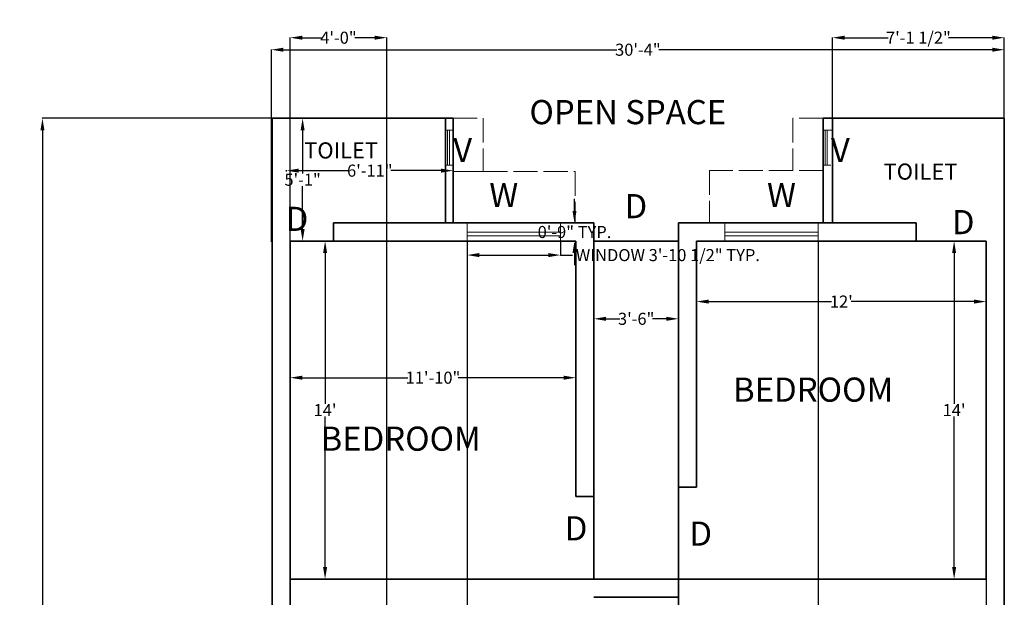
# Model space of a CAD drawing. Units: inches. Extents: x -732 to -187, y 754 to 1605.
# Tile 2 of 2: x -732 to -242, y 1318 to 1605. Entities that reach past the tile are written whole.
import ezdxf

# ---------------------------------------------------------------- set-up
doc = ezdxf.new("R2010")
doc.units = ezdxf.units.IN
doc.header["$MEASUREMENT"] = 0
doc.linetypes.add('ACAD_ISO02W100', pattern=[15, 12, -3])
for name, color, linetype, lineweight in [('A-ANNO-DIMS', 2, 'Continuous', 18), ('A-ANNO-TEXT', 3, 'Continuous', 18), ('A-AREA-IDEN', 7, 'Continuous', 25), ('A-GLAZ', 4, 'Continuous', 18), ('A-ROOF', 8, 'Continuous', 18), ('A-ROOF-OVHD', 8, 'ACAD_ISO02W100', 18), ('A-WALL', 7, 'Continuous', 35)]:
    doc.layers.add(name, color=color, linetype=linetype, lineweight=lineweight)
doc.styles.get("Standard").update_dxf_attribs({"font": 'arial.ttf'})
doc.dimstyles.get("Standard").update_dxf_attribs({"dimtxt": 6, "dimasz": 6, "dimexe": 0.18, "dimexo": 0.0625, "dimgap": 0.09, "dimtad": 0, "dimtih": 1, "dimtoh": 1, "dimdec": 0, "dimzin": 0, "dimdsep": 46, "dimlunit": 3, "dimtxsty": 'Standard', "dimcen": 0.09, "dimadec": 0, "dimazin": 0, "dimtfac": 1, "dimtdec": 0, "dimtofl": 0, "dimtmove": 0, "dimatfit": 3, "dimfxl": 1, "dimtolj": 1, "dimtzin": 0, "dimarcsym": 0})

# ---------------------------------------------------------------- blocks, each defined once
blk = doc.blocks.new('*D1')
at = {"layer": 'A-ANNO-DIMS', "color": 0, "lineweight": -2, "transparency": 16777216}
for p, q in [((-446.28, 1440.67), (-446.28, 1456.43)), ((-440.28, 1456.25), (-433.34, 1456.25)), ((-410.28, 1456.25), (-417.22, 1456.25)), ((-404.28, 1440.67), (-404.28, 1456.43))]:
    blk.add_line(p, q, dxfattribs=at)
at = {"layer": 'A-ANNO-DIMS', "color": 0, "transparency": 16777216}
for points in [[(-440.28, 1457.25), (-440.28, 1455.25), (-446.28, 1456.25)], [(-410.28, 1457.25), (-410.28, 1455.25), (-404.28, 1456.25)]]:
    blk.add_solid(points, dxfattribs=at)
at = {"layer": 'Defpoints', "color": 0, "transparency": 16777216}
for p in [(-404.28, 1456.25), (-446.28, 1440.61), (-404.28, 1440.61)]:
    blk.add_point(p, dxfattribs=at)
at = {"layer": 'A-ANNO-DIMS', "color": 0, "transparency": 16777216, "insert": (-425.28, 1456.25), "char_height": 6, "attachment_point": 5}
blk.add_mtext('\\A1;3\'-6"', dxfattribs=at)
blk = doc.blocks.new('*D2')
at = {"layer": 'A-ANNO-DIMS', "color": 0, "lineweight": -2, "transparency": 16777216}
for p, q in [((-395.28, 1479.29), (-395.28, 1464.63)), ((-251.28, 1479.29), (-251.28, 1464.63)), ((-389.28, 1464.81), (-328.18, 1464.81)), ((-257.28, 1464.81), (-318.38, 1464.81))]:
    blk.add_line(p, q, dxfattribs=at)
at = {"layer": 'A-ANNO-DIMS', "color": 0, "transparency": 16777216}
for points in [[(-389.28, 1465.81), (-389.28, 1463.81), (-395.28, 1464.81)], [(-257.28, 1465.81), (-257.28, 1463.81), (-251.28, 1464.81)]]:
    blk.add_solid(points, dxfattribs=at)
at = {"layer": 'Defpoints', "color": 0, "transparency": 16777216}
for p in [(-395.28, 1479.35), (-251.28, 1479.35), (-251.28, 1464.81)]:
    blk.add_point(p, dxfattribs=at)
at = {"layer": 'A-ANNO-DIMS', "color": 0, "transparency": 16777216, "insert": (-323.28, 1464.81), "char_height": 6, "attachment_point": 5}
blk.add_mtext("\\A1;12'", dxfattribs=at)
blk = doc.blocks.new('*D3')
at = {"layer": 'A-ANNO-DIMS', "color": 0, "lineweight": -2, "transparency": 16777216}
for p, q in [((-597.28, 1427.05), (-597.28, 1427.17)), ((-591.28, 1426.99), (-538.72, 1426.99)), ((-461.28, 1426.99), (-513.83, 1426.99)), ((-455.28, 1427.05), (-455.28, 1427.17))]:
    blk.add_line(p, q, dxfattribs=at)
at = {"layer": 'A-ANNO-DIMS', "color": 0, "transparency": 16777216}
for points in [[(-591.28, 1427.99), (-591.28, 1425.99), (-597.28, 1426.99)], [(-461.28, 1427.99), (-461.28, 1425.99), (-455.28, 1426.99)]]:
    blk.add_solid(points, dxfattribs=at)
at = {"layer": 'Defpoints', "color": 0, "transparency": 16777216}
for p in [(-597.28, 1426.99), (-455.28, 1426.99), (-455.28, 1426.99)]:
    blk.add_point(p, dxfattribs=at)
at = {"layer": 'A-ANNO-DIMS', "color": 0, "transparency": 16777216, "insert": (-526.28, 1426.99), "char_height": 6, "attachment_point": 5}
blk.add_mtext('\\A1;11\'-10"', dxfattribs=at)
blk = doc.blocks.new('*D19')
at = {"layer": 'A-ANNO-DIMS', "color": 0, "lineweight": -2, "transparency": 16777216}
for p, q in [((-251.34, 1494.88), (-267.41, 1494.88)), ((-267.23, 1488.88), (-267.23, 1413.98)), ((-267.23, 1332.88), (-267.23, 1407.78)), ((-251.34, 1326.88), (-267.41, 1326.88))]:
    blk.add_line(p, q, dxfattribs=at)
at = {"layer": 'A-ANNO-DIMS', "color": 0, "transparency": 16777216}
for points in [[(-268.23, 1488.88), (-266.23, 1488.88), (-267.23, 1494.88)], [(-268.23, 1332.88), (-266.23, 1332.88), (-267.23, 1326.88)]]:
    blk.add_solid(points, dxfattribs=at)
at = {"layer": 'Defpoints', "color": 0, "transparency": 16777216}
for p in [(-251.28, 1494.88), (-267.23, 1326.88), (-251.28, 1326.88)]:
    blk.add_point(p, dxfattribs=at)
at = {"layer": 'A-ANNO-DIMS', "color": 0, "transparency": 16777216, "insert": (-267.23, 1410.88), "char_height": 6, "attachment_point": 5}
blk.add_mtext("\\A1;14'", dxfattribs=at)
blk = doc.blocks.new('*D20')
at = {"layer": 'A-ANNO-DIMS', "color": 0, "lineweight": -2, "transparency": 16777216}
for p, q in [((-597.22, 1494.88), (-579.74, 1494.88)), ((-579.92, 1488.88), (-579.92, 1413.98)), ((-579.92, 1332.88), (-579.92, 1407.77)), ((-597.22, 1326.88), (-579.74, 1326.88))]:
    blk.add_line(p, q, dxfattribs=at)
at = {"layer": 'A-ANNO-DIMS', "color": 0, "transparency": 16777216}
for points in [[(-580.92, 1488.88), (-578.92, 1488.88), (-579.92, 1494.88)], [(-580.92, 1332.88), (-578.92, 1332.88), (-579.92, 1326.88)]]:
    blk.add_solid(points, dxfattribs=at)
at = {"layer": 'Defpoints', "color": 0, "transparency": 16777216}
for p in [(-597.28, 1494.88), (-597.28, 1326.88), (-579.92, 1326.88)]:
    blk.add_point(p, dxfattribs=at)
at = {"layer": 'A-ANNO-DIMS', "color": 0, "transparency": 16777216, "insert": (-579.92, 1410.88), "char_height": 6, "attachment_point": 5}
blk.add_mtext("\\A1;14'", dxfattribs=at)
blk = doc.blocks.new('*D21')
at = {"layer": 'A-ANNO-DIMS', "color": 0, "lineweight": -2, "transparency": 16777216}
for p, q in [((-584.99, 1555.88), (-591.28, 1555.88)), ((-591.1, 1549.88), (-591.1, 1528.53)), ((-591.1, 1500.88), (-591.1, 1522.22)), ((-584.99, 1494.88), (-591.28, 1494.88))]:
    blk.add_line(p, q, dxfattribs=at)
at = {"layer": 'A-ANNO-DIMS', "color": 0, "transparency": 16777216}
for points in [[(-592.1, 1549.88), (-590.1, 1549.88), (-591.1, 1555.88)], [(-592.1, 1500.88), (-590.1, 1500.88), (-591.1, 1494.88)]]:
    blk.add_solid(points, dxfattribs=at)
at = {"layer": 'Defpoints', "color": 0, "transparency": 16777216}
for p in [(-584.93, 1555.88), (-591.1, 1494.88), (-584.93, 1494.88)]:
    blk.add_point(p, dxfattribs=at)
at = {"layer": 'A-ANNO-DIMS', "color": 0, "transparency": 16777216, "insert": (-591.1, 1525.38), "char_height": 6, "attachment_point": 5}
blk.add_mtext('\\A1;5\'-1"', dxfattribs=at)
blk = doc.blocks.new('*D22')
at = {"layer": 'A-ANNO-DIMS', "color": 0, "lineweight": -2, "transparency": 16777216}
for p, q in [((-599.1, 1529.44), (-599.1, 1530.06)), ((-593.1, 1529.88), (-568.1, 1529.88)), ((-522.28, 1529.88), (-547.28, 1529.88)), ((-516.28, 1529.44), (-516.28, 1530.06))]:
    blk.add_line(p, q, dxfattribs=at)
at = {"layer": 'A-ANNO-DIMS', "color": 0, "transparency": 16777216}
for points in [[(-593.1, 1530.88), (-593.1, 1528.88), (-599.1, 1529.88)], [(-522.28, 1530.88), (-522.28, 1528.88), (-516.28, 1529.88)]]:
    blk.add_solid(points, dxfattribs=at)
at = {"layer": 'Defpoints', "color": 0, "transparency": 16777216}
for p in [(-599.1, 1529.88), (-599.1, 1529.38), (-516.28, 1529.38)]:
    blk.add_point(p, dxfattribs=at)
at = {"layer": 'A-ANNO-DIMS', "color": 0, "transparency": 16777216, "insert": (-557.69, 1529.88), "char_height": 6, "attachment_point": 5}
blk.add_mtext('\\A1;6\'-11"', dxfattribs=at)
blk = doc.blocks.new('*D23')
at = {"layer": 'A-ANNO-DIMS', "color": 0, "lineweight": -2, "transparency": 16777216}
for p, q in [((-606.6, 1494.55), (-606.6, 1590.14)), ((-600.6, 1589.96), (-434.83, 1589.96)), ((-248.28, 1589.96), (-414.04, 1589.96)), ((-242.28, 1494.55), (-242.28, 1590.14))]:
    blk.add_line(p, q, dxfattribs=at)
at = {"layer": 'A-ANNO-DIMS', "color": 0, "transparency": 16777216}
for points in [[(-600.6, 1590.96), (-600.6, 1588.96), (-606.6, 1589.96)], [(-248.28, 1590.96), (-248.28, 1588.96), (-242.28, 1589.96)]]:
    blk.add_solid(points, dxfattribs=at)
at = {"layer": 'Defpoints', "color": 0, "transparency": 16777216}
for p in [(-242.28, 1589.96), (-606.6, 1494.48), (-242.28, 1494.48)]:
    blk.add_point(p, dxfattribs=at)
at = {"layer": 'A-ANNO-DIMS', "color": 0, "transparency": 16777216, "insert": (-424.44, 1589.96), "char_height": 6, "attachment_point": 5}
blk.add_mtext('\\A1;30\'-4"', dxfattribs=at)
blk = doc.blocks.new('*D24')
at = {"layer": 'A-ANNO-DIMS', "color": 0, "lineweight": -2, "transparency": 16777216}
for p, q in [((-606.34, 1555.88), (-720.61, 1555.88)), ((-720.43, 1549.88), (-720.43, 1197.03)), ((-720.43, 837.88), (-720.43, 1190.72)), ((-606.34, 831.88), (-720.61, 831.88))]:
    blk.add_line(p, q, dxfattribs=at)
at = {"layer": 'A-ANNO-DIMS', "color": 0, "transparency": 16777216}
for points in [[(-721.43, 1549.88), (-719.43, 1549.88), (-720.43, 1555.88)], [(-721.43, 837.88), (-719.43, 837.88), (-720.43, 831.88)]]:
    blk.add_solid(points, dxfattribs=at)
at = {"layer": 'Defpoints', "color": 0, "transparency": 16777216}
for p in [(-606.28, 1555.88), (-720.43, 831.88), (-606.28, 831.88)]:
    blk.add_point(p, dxfattribs=at)
at = {"layer": 'A-ANNO-DIMS', "color": 0, "transparency": 16777216, "insert": (-720.43, 1193.88), "char_height": 6, "attachment_point": 5}
blk.add_mtext('\\A1;60\'-4"', dxfattribs=at)
blk = doc.blocks.new('WIN-REAR-BEDROOM')
for p, q in [((0, 9), (0, 0)), ((46.43, 9), (46.43, 0)), ((0, 4.5), (46.43, 4.5)), ((0, 2.55), (46.43, 2.55))]:
    blk.add_line(p, q)
blk = doc.blocks.new('*D26')
at = {"layer": 'A-ANNO-DIMS', "color": 0, "lineweight": -2, "transparency": 16777216}
for p, q in [((-509.33, 1494.81), (-509.33, 1487.73)), ((-462.9, 1494.81), (-462.9, 1487.73)), ((-503.33, 1487.91), (-468.9, 1487.91)), ((-462.9, 1487.91), (-456.9, 1487.91))]:
    blk.add_line(p, q, dxfattribs=at)
at = {"layer": 'A-ANNO-DIMS', "color": 0, "transparency": 16777216}
for points in [[(-503.33, 1488.91), (-503.33, 1486.91), (-509.33, 1487.91)], [(-468.9, 1488.91), (-468.9, 1486.91), (-462.9, 1487.91)]]:
    blk.add_solid(points, dxfattribs=at)
at = {"layer": 'Defpoints', "color": 0, "transparency": 16777216}
for p in [(-509.33, 1494.88), (-462.9, 1494.88), (-462.9, 1487.91)]:
    blk.add_point(p, dxfattribs=at)
at = {"layer": 'A-ANNO-DIMS', "color": 0, "transparency": 16777216, "insert": (-409.53, 1487.91), "char_height": 6, "attachment_point": 5}
blk.add_mtext('\\A1;WINDOW 3\'-10 1/2" TYP.', dxfattribs=at)
blk = doc.blocks.new('*D27')
at = {"layer": 'A-ANNO-DIMS', "color": 0, "lineweight": -2, "transparency": 16777216}
for p, q in [((-455.94, 1509.88), (-455.94, 1515.88)), ((-462.84, 1503.88), (-455.76, 1503.88)), ((-462.84, 1494.88), (-455.76, 1494.88)), ((-455.94, 1488.88), (-455.94, 1482.88))]:
    blk.add_line(p, q, dxfattribs=at)
at = {"layer": 'A-ANNO-DIMS', "color": 0, "transparency": 16777216}
for points in [[(-456.94, 1509.88), (-454.94, 1509.88), (-455.94, 1503.88)], [(-456.94, 1488.88), (-454.94, 1488.88), (-455.94, 1494.88)]]:
    blk.add_solid(points, dxfattribs=at)
at = {"layer": 'Defpoints', "color": 0, "transparency": 16777216}
for p in [(-462.9, 1503.88), (-455.94, 1503.88), (-462.9, 1494.88)]:
    blk.add_point(p, dxfattribs=at)
at = {"layer": 'A-ANNO-DIMS', "color": 0, "transparency": 16777216, "insert": (-455.94, 1499.38), "char_height": 6, "attachment_point": 5}
blk.add_mtext('\\A1;0\'-9" TYP.', dxfattribs=at)
blk = doc.blocks.new('*D33')
at = {"layer": 'A-ANNO-DIMS', "color": 0, "lineweight": -2, "transparency": 16777216}
for p, q in [((-597.28, 1084.94), (-597.28, 1596.11)), ((-591.28, 1595.93), (-581.46, 1595.93)), ((-555.28, 1595.93), (-565.09, 1595.93)), ((-549.28, 1084.94), (-549.28, 1596.11))]:
    blk.add_line(p, q, dxfattribs=at)
at = {"layer": 'A-ANNO-DIMS', "color": 0, "transparency": 16777216}
for points in [[(-591.28, 1596.93), (-591.28, 1594.93), (-597.28, 1595.93)], [(-555.28, 1596.93), (-555.28, 1594.93), (-549.28, 1595.93)]]:
    blk.add_solid(points, dxfattribs=at)
at = {"layer": 'Defpoints', "color": 0, "transparency": 16777216}
for p in [(-549.28, 1595.93), (-597.28, 1084.88), (-549.28, 1084.88)]:
    blk.add_point(p, dxfattribs=at)
at = {"layer": 'A-ANNO-DIMS', "color": 0, "transparency": 16777216, "insert": (-573.28, 1595.93), "char_height": 6, "attachment_point": 5}
blk.add_mtext('\\A1;4\'-0"', dxfattribs=at)
blk = doc.blocks.new('*D36')
at = {"layer": 'A-ANNO-DIMS', "color": 0, "lineweight": -2, "transparency": 16777216}
for p, q in [((-327.69, 1555.94), (-327.69, 1596.11)), ((-321.69, 1595.93), (-300.02, 1595.93)), ((-248.28, 1595.93), (-269.95, 1595.93)), ((-242.28, 1555.94), (-242.28, 1596.11))]:
    blk.add_line(p, q, dxfattribs=at)
at = {"layer": 'A-ANNO-DIMS', "color": 0, "transparency": 16777216}
for points in [[(-321.69, 1596.93), (-321.69, 1594.93), (-327.69, 1595.93)], [(-248.28, 1596.93), (-248.28, 1594.93), (-242.28, 1595.93)]]:
    blk.add_solid(points, dxfattribs=at)
at = {"layer": 'Defpoints', "color": 0, "transparency": 16777216}
for p in [(-242.28, 1595.93), (-327.69, 1555.88), (-242.28, 1555.88)]:
    blk.add_point(p, dxfattribs=at)
at = {"layer": 'A-ANNO-DIMS', "color": 0, "transparency": 16777216, "insert": (-284.98, 1595.93), "char_height": 6, "attachment_point": 5}
blk.add_mtext('\\A1;7\'-1 1/2"', dxfattribs=at)
blk = doc.blocks.new('*D37')
at = {"layer": 'A-ANNO-DIMS', "color": 0, "lineweight": -2, "transparency": 16777216}
for p, q in [((-597.28, 1494.81), (-597.28, 763.13)), ((-509.33, 1494.81), (-509.33, 763.13)), ((-591.28, 763.31), (-561.35, 763.31)), ((-515.33, 763.31), (-545.27, 763.31))]:
    blk.add_line(p, q, dxfattribs=at)
at = {"layer": 'A-ANNO-DIMS', "color": 0, "transparency": 16777216}
for points in [[(-591.28, 764.31), (-591.28, 762.31), (-597.28, 763.31)], [(-515.33, 764.31), (-515.33, 762.31), (-509.33, 763.31)]]:
    blk.add_solid(points, dxfattribs=at)
at = {"layer": 'Defpoints', "color": 0, "transparency": 16777216}
for p in [(-597.28, 1494.88), (-509.33, 1494.88), (-509.33, 763.31)]:
    blk.add_point(p, dxfattribs=at)
at = {"layer": 'A-ANNO-DIMS', "color": 0, "transparency": 16777216, "insert": (-553.31, 763.31), "char_height": 6, "attachment_point": 5}
blk.add_mtext('\\A1;7\'-4"', dxfattribs=at)
blk = doc.blocks.new('*D38')
at = {"layer": 'A-ANNO-DIMS', "color": 0, "lineweight": -2, "transparency": 16777216}
for p, q in [((-334.82, 1494.81), (-334.82, 763.13)), ((-251.28, 1494.82), (-251.28, 763.13)), ((-328.82, 763.31), (-310.45, 763.31)), ((-257.28, 763.31), (-275.65, 763.31))]:
    blk.add_line(p, q, dxfattribs=at)
at = {"layer": 'A-ANNO-DIMS', "color": 0, "transparency": 16777216}
for points in [[(-328.82, 764.31), (-328.82, 762.31), (-334.82, 763.31)], [(-257.28, 764.31), (-257.28, 762.31), (-251.28, 763.31)]]:
    blk.add_solid(points, dxfattribs=at)
at = {"layer": 'Defpoints', "color": 0, "transparency": 16777216}
for p in [(-334.82, 1494.88), (-251.28, 1494.88), (-251.28, 763.31)]:
    blk.add_point(p, dxfattribs=at)
at = {"layer": 'A-ANNO-DIMS', "color": 0, "transparency": 16777216, "insert": (-293.05, 763.31), "char_height": 6, "attachment_point": 5}
blk.add_mtext('\\A1;6\'-11 1/2"', dxfattribs=at)

msp = doc.modelspace()

# ---------------------------------------------------------------- linework, layer by layer
at = {"layer": 'A-GLAZ'}
for p, q in [((-520, 1549.98), (-516.28, 1549.98)), ((-519.04, 1549.98), (-519.04, 1532.62)), ((-518.05, 1549.98), (-518.14, 1532.62)), ((-332.23, 1549.98), (-327.69, 1549.98)), ((-331.27, 1549.98), (-331.27, 1532.62)), ((-330.28, 1549.98), (-330.37, 1532.62)), ((-520, 1532.62), (-516.28, 1532.62)), ((-332.23, 1532.62), (-328.51, 1532.62))]:
    msp.add_line(p, q, dxfattribs=at)
at = {"layer": 'A-ROOF'}
msp.add_line((-501.27, 1529.38), (-516.28, 1529.38), dxfattribs=at)
at = {"layer": 'A-ROOF-OVHD'}
for p, q in [((-516.28, 1555.88), (-501.27, 1555.88)), ((-501.27, 1555.88), (-501.27, 1529.38)), ((-332.28, 1555.88), (-347.36, 1555.88)), ((-347.36, 1555.88), (-347.36, 1529.88)), ((-516.28, 1529.38), (-455.67, 1529.38)), ((-455.67, 1529.38), (-455.67, 1503.88)), ((-379.11, 1529.88), (-388.9, 1529.88)), ((-388.9, 1529.88), (-388.9, 1503.88)), ((-332.28, 1529.88), (-379.11, 1529.88))]:
    msp.add_line(p, q, dxfattribs=at)
at = {"layer": 'A-WALL'}
for p, q in [((-606.28, 1555.88), (-516.28, 1555.88)), ((-606.28, 1503.88), (-606.28, 1555.88)), ((-516.28, 1555.88), (-520, 1555.88)), ((-520, 1555.88), (-520, 1503.88)), ((-516.28, 1555.88), (-516.28, 1503.88)), ((-242.28, 1555.88), (-332.28, 1555.88)), ((-332.28, 1555.88), (-332.28, 1503.88)), ((-327.69, 1555.88), (-327.69, 1503.88)), ((-242.28, 1503.88), (-242.28, 1555.88)), ((-606.28, 1326.88), (-606.28, 1503.88)), ((-516.28, 1503.88), (-575.75, 1503.88)), ((-575.75, 1503.88), (-575.75, 1494.88)), ((-575.75, 1503.88), (-446.28, 1503.88)), ((-520, 1503.88), (-516.28, 1503.88)), ((-446.28, 1503.88), (-446.28, 1494.88)), ((-404.28, 1503.88), (-286.13, 1503.88)), ((-404.28, 1317.88), (-404.28, 1503.88)), ((-286.13, 1503.88), (-286.13, 1494.88)), ((-242.28, 1503.88), (-242.28, 1326.88)), ((-597.28, 1494.88), (-455.28, 1494.88)), ((-597.28, 1326.88), (-597.28, 1494.88)), ((-455.28, 1494.88), (-588.28, 1494.88)), ((-455.28, 1368.04), (-455.28, 1494.88)), ((-446.28, 1494.88), (-446.28, 1326.88)), ((-446.28, 1494.88), (-404.28, 1494.88)), ((-446.28, 1326.88), (-446.28, 1494.88)), ((-404.28, 1494.88), (-404.28, 1326.88)), ((-395.28, 1372.67), (-395.28, 1494.88)), ((-395.28, 1494.88), (-251.28, 1494.88)), ((-251.28, 1494.88), (-251.28, 1326.88)), ((-404.28, 1372.67), (-395.28, 1372.67)), ((-446.28, 1368.04), (-455.28, 1368.04)), ((-606.28, 1326.88), (-606.28, 831.88)), ((-446.28, 1326.88), (-597.28, 1326.88)), ((-404.28, 1326.88), (-446.28, 1326.88)), ((-251.28, 1326.88), (-404.28, 1326.88)), ((-242.28, 1326.88), (-242.28, 831.88)), ((-404.28, 1317.88), (-446.28, 1317.88)), ((-404.28, 1317.88), (-404.28, 1032.88))]:
    msp.add_line(p, q, dxfattribs=at)

# ---------------------------------------------------------------- block references
at = {"layer": 'A-GLAZ'}
for p in [(-509.33, 1494.88), (-381.25, 1494.88)]:
    msp.add_blockref('WIN-REAR-BEDROOM', p, dxfattribs=at)

# ---------------------------------------------------------------- texts
at = {"layer": 'A-ANNO-TEXT', "char_height": 12}
for s, width, insert, attachment_point in [('V', 35.4038, (-516.26, 1546.14), 1), ('V', 35.4038, (-328.49, 1546.14), 1), ('W', 35.4038, (-498.3, 1523.76), 1), ('W', 35.4038, (-345.85, 1523.76), 3), ('D', 8.414, (-431.06, 1518.24), 1), ('D', 8.414, (-599.52, 1511.9), 1), ('D', 8.414, (-268.34, 1510.3), 1), ('D', 8.414, (-460.77, 1358.15), 1), ('D', 8.414, (-398.83, 1355.51), 1)]:
    msp.add_mtext_dynamic_manual_height_columns(s, width=width, gutter_width=1, heights=[0], dxfattribs=dict(at, insert=insert, attachment_point=attachment_point))
at = {"layer": 'A-AREA-IDEN', "attachment_point": 1}
for s, width, insert, char_height in [('OPEN SPACE', 110.1239, (-478.34, 1564.95), 12), ('TOILET', 13.784, (-590.32, 1543.92), 8), ('TOILET', 13.784, (-302.3, 1533.4), 8), ('BEDROOM', 76.222, (-377.12, 1427.06), 12), ('BEDROOM', 76.222, (-582.17, 1402.69), 12)]:
    msp.add_mtext_dynamic_manual_height_columns(s, width=width, gutter_width=1, heights=[0], dxfattribs=dict(at, insert=insert, char_height=char_height))

# ---------------------------------------------------------------- dimensions: what is measured, and where the dimension line sits
at = {"layer": 'A-ANNO-DIMS'}
for base, p1, p2, override, picture, middle in [((-242.28, 1595.93), (-327.69, 1555.88), (-242.28, 1555.88), {"dimdec": 1, "dimlfac": 1, "dimrnd": 0, "dimzin": 1, "dimdsep": 46, "dimlunit": 4, "dimfrac": 2}, '*D36', (-284.98, 1595.93)), ((-549.28, 1595.93), (-597.28, 1084.88), (-549.28, 1084.88), {"dimdec": 1, "dimlfac": 1, "dimrnd": 0, "dimzin": 1, "dimdsep": 46, "dimlunit": 4, "dimfrac": 2}, '*D33', (-573.28, 1595.93)), ((-242.28, 1589.96), (-606.6, 1494.48), (-242.28, 1494.48), {"dimclrd": 0, "dimclre": 0, "dimclrt": 0}, '*D23', (-424.44, 1589.96)), ((-599.1, 1529.88), (-516.28, 1529.38), (-599.1, 1529.38), {"dimclrd": 0, "dimclre": 0, "dimclrt": 0}, '*D22', (-557.69, 1529.88)), ((-509.3331, 763.3082), (-597.2785, 1494.8762), (-509.3331, 1494.8762), {"dimdec": 1, "dimlfac": 1, "dimrnd": 0, "dimzin": 1, "dimdsep": 46, "dimlunit": 4, "dimfrac": 2}, '*D37', (-553.3058, 763.3082)), ((-251.28, 763.31), (-334.82, 1494.88), (-251.28, 1494.88), {"dimdec": 1, "dimlfac": 1, "dimrnd": 0, "dimzin": 1, "dimdsep": 46, "dimlunit": 4, "dimfrac": 2}, '*D38', (-293.05, 763.31)), ((-251.28, 1464.81), (-395.28, 1479.35), (-251.28, 1479.35), {"dimclrd": 0, "dimclre": 0, "dimclrt": 0}, '*D2', (-323.28, 1464.81)), ((-404.28, 1456.25), (-446.28, 1440.61), (-404.28, 1440.61), {"dimclrd": 0, "dimclre": 0, "dimclrt": 0}, '*D1', (-425.28, 1456.25)), ((-455.28, 1426.99), (-597.28, 1426.99), (-455.28, 1426.99), {"dimclrd": 0, "dimclre": 0, "dimclrt": 0}, '*D3', (-526.28, 1426.99))]:
    dim = msp.add_linear_dim(base=base, p1=p1, p2=p2, dimstyle='Standard', override=override, dxfattribs=at)
    dim.commit()
    dim.dimension.update_dxf_attribs({"geometry": picture, "text_midpoint": middle})
for base, p1, p2, picture, middle in [((-720.43, 831.88), (-606.28, 1555.88), (-606.28, 831.88), '*D24', (-720.43, 1193.88)), ((-591.1, 1494.88), (-584.93, 1555.88), (-584.93, 1494.88), '*D21', (-591.1, 1525.38)), ((-579.92, 1326.88), (-597.28, 1494.88), (-597.28, 1326.88), '*D20', (-579.92, 1410.88)), ((-267.23, 1326.88), (-251.28, 1494.88), (-251.28, 1326.88), '*D19', (-267.23, 1410.88))]:
    dim = msp.add_linear_dim(base=base, p1=p1, p2=p2, angle=90, dimstyle='Standard', override={"dimclrd": 0, "dimclre": 0, "dimclrt": 0}, dxfattribs=at)
    dim.commit()
    dim.dimension.update_dxf_attribs({"geometry": picture, "text_midpoint": middle})
dim = msp.add_linear_dim(base=(-455.94, 1503.88), p1=(-462.9, 1494.88), p2=(-462.9, 1503.88), angle=90, text='<> TYP.', dimstyle='Standard', override={"dimdec": 1, "dimlfac": 1, "dimrnd": 0, "dimzin": 1, "dimdsep": 46, "dimlunit": 4, "dimfrac": 2}, dxfattribs=at)
dim.commit()
dim.dimension.update_dxf_attribs({"geometry": '*D27', "text_midpoint": (-455.94, 1499.38)})
dim = msp.add_linear_dim(base=(-462.9, 1487.91), p1=(-509.33, 1494.88), p2=(-462.9, 1494.88), text='WINDOW <> TYP.', dimstyle='Standard', override={"dimdec": 1, "dimlfac": 1, "dimrnd": 0, "dimzin": 1, "dimdsep": 46, "dimlunit": 4, "dimfrac": 2}, dxfattribs=at)
dim.commit()
dim.dimension.update_dxf_attribs({"geometry": '*D26', "text_midpoint": (-409.53, 1487.91)})

doc.saveas('drawing.dxf')
